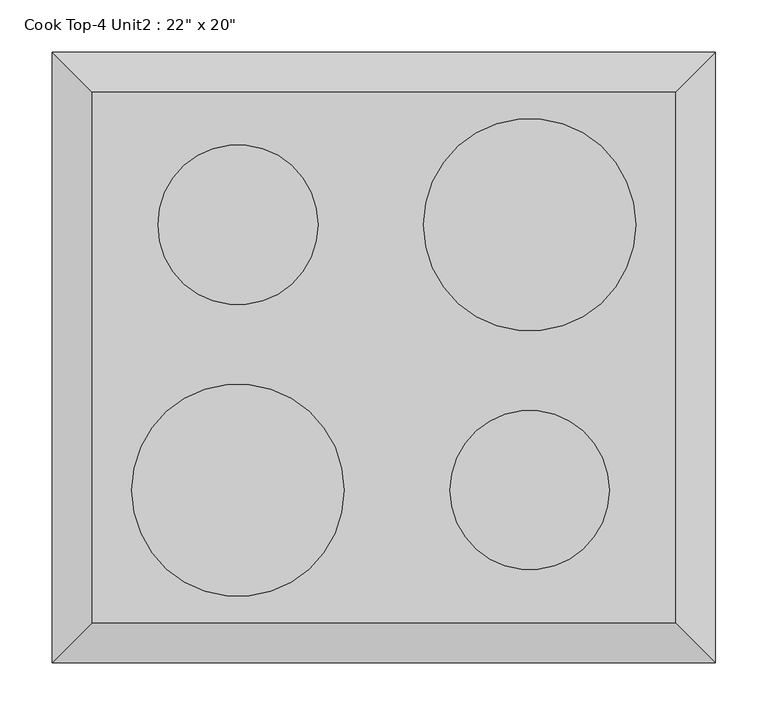
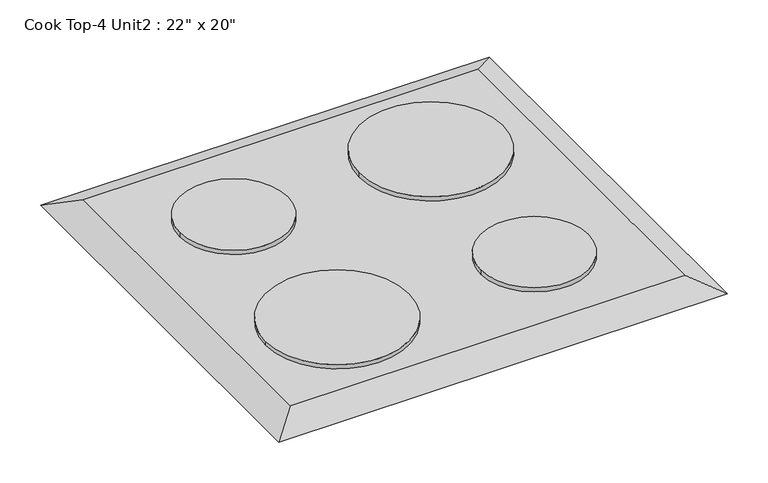
"""IFC4 building model written with IfcOpenShell, lengths in millimetres: proxy geometry."""

from ifc_helpers import new_model, si_unit, point, frame, frame_2d, origin, place, context, project, spatial, circle_curve, trimmed, segment, composite_curve, outline, extrude, faceted_brep, source, transform, mapped, element, save


def proxy_a6faaae8(model_context):
    return source(origin(), model_context, "Body", "SolidModel", [
        extrude(outline(composite_curve([segment(trimmed(circle_curve(frame_2d((-139.7, 127.0)), 76.5869489), [point((-63.1130511, 127.0))], [point((-216.2869489, 127.0))], False, "CARTESIAN"), True, "CONTINUOUS"), segment(trimmed(circle_curve(frame_2d((-139.7, 127.0)), 76.5869489), [point((-216.2869489, 127.0))], [point((-63.1130511, 127.0))], False, "CARTESIAN"), True, "CONTINUOUS")], self_intersect=False)), frame((0.0, 0.0, 918.0), z_axis=(0.0, 0.0, 1.0), x_axis=(1.0, 0.0, 0.0)), (0.0, 0.0, 1.0), 6.35),
        extrude(outline(composite_curve([segment(trimmed(circle_curve(frame_2d((139.7, -127.0)), 76.2), [point((215.9, -127.0))], [point((63.5, -127.0))], False, "CARTESIAN"), True, "CONTINUOUS"), segment(trimmed(circle_curve(frame_2d((139.7, -127.0)), 76.2), [point((63.5, -127.0))], [point((215.9, -127.0))], False, "CARTESIAN"), True, "CONTINUOUS")], self_intersect=False)), frame((0.0, 0.0, 918.0), z_axis=(0.0, 0.0, 1.0), x_axis=(1.0, 0.0, 0.0)), (0.0, 0.0, 1.0), 6.35),
        extrude(outline(composite_curve([segment(trimmed(circle_curve(frame_2d((139.7, 127.0)), 101.6), [point((38.1, 127.0))], [point((241.3, 127.0))], False, "CARTESIAN"), True, "CONTINUOUS"), segment(trimmed(circle_curve(frame_2d((139.7, 127.0)), 101.6), [point((241.3, 127.0))], [point((38.1, 127.0))], False, "CARTESIAN"), True, "CONTINUOUS")], self_intersect=False)), frame((0.0, 0.0, 918.0), z_axis=(0.0, 0.0, 1.0), x_axis=(1.0, 0.0, 0.0)), (0.0, 0.0, 1.0), 6.35),
        faceted_brep([(279.4, 254.0, 918.0), (-279.4, 254.0, 918.0), (-279.4, -254.0, 918.0), (279.4, -254.0, 918.0), (317.5, 292.1, 900.0), (317.5, -292.1, 900.0), (-317.5, -292.1, 900.0), (-317.5, 292.1, 900.0)], [[[0, 1, 2, 3]], [[4, 5, 6, 7]], [[4, 7, 1, 0]], [[7, 6, 2, 1]], [[6, 5, 3, 2]], [[5, 4, 0, 3]]]),
        extrude(outline(composite_curve([segment(trimmed(circle_curve(frame_2d((-139.7, -127.0)), 101.6), [point((-38.1, -127.0))], [point((-241.3, -127.0))], False, "CARTESIAN"), True, "CONTINUOUS"), segment(trimmed(circle_curve(frame_2d((-139.7, -127.0)), 101.6), [point((-241.3, -127.0))], [point((-38.1, -127.0))], False, "CARTESIAN"), True, "CONTINUOUS")], self_intersect=False)), frame((0.0, 0.0, 918.0), z_axis=(0.0, 0.0, 1.0), x_axis=(1.0, 0.0, 0.0)), (0.0, 0.0, 1.0), 6.35),
    ])


if __name__ == "__main__":
    model = new_model("IFC4")
    model_context = context("Model", 3, world=origin())
    ifc_project = project(units=[si_unit("LENGTHUNIT", "METRE", prefix="MILLI")], contexts=[model_context])
    site = spatial("IfcSite", under=ifc_project)
    building = spatial("IfcBuilding", under=site)
    placement = place(None, origin())
    proxy_shape = proxy_a6faaae8(model_context)
    element("IfcBuildingElementProxy", 1, Name="Cook Top-4 Unit2 : 22\" x 20\"", ObjectType="Cook Top-4 Unit2 : 22\" x 20\"", at=placement, inside=building, context=model_context, shape_type="MappedRepresentation", body=[
        mapped(proxy_shape, transform((0.0, 0.0, 0.0), x_axis=(1.0, 0.0, 0.0), y_axis=(0.0, 1.0, 0.0), z_axis=(0.0, 0.0, 1.0))),
    ])
    save(model, "model.ifc")

# Revit data of these elements
# Type "Cook Top-4 Unit2 : 22\" x 20\""
#   Depth = 1' - 8"
#   Width = 1' - 10"
#   Burner Material = Steel, Chrome Plated
#   Cooktop Material = Steel, Polished
#   Default Elevation = 0
#   Assembly Code = ""
# Element 1 (IfcBuildingElementProxy, "Cook Top-4 Unit2 : 22\" x 20\"")
#   Materials on its faces: "Steel, Chrome Plated", "Steel, Polished"
# Materials
#   "Steel, Chrome Plated": class "Metal", colour RGB 17 17 17, transparency 0, Description = "Chromiuim plated steel", Cost = 0
#   "Steel, Polished": class "Metal", colour RGB 57 57 57, transparency 0, Description = "Polished steel", Cost = 0
